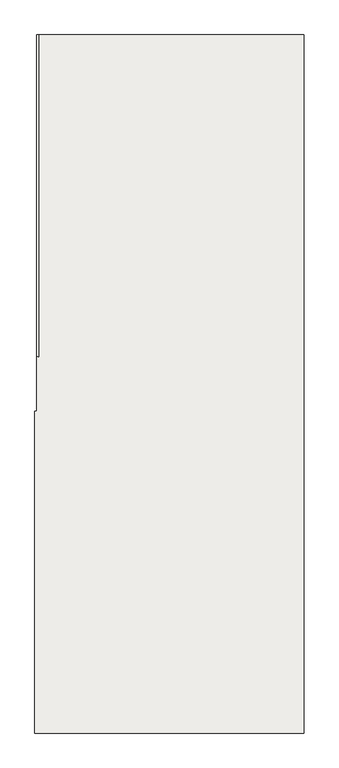
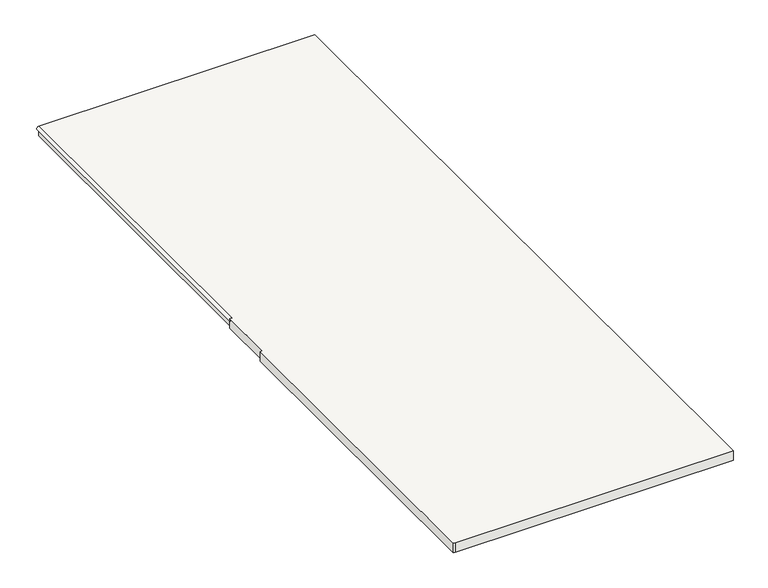
"""IFC4 building model written with IfcOpenShell, lengths in millimetres: slab geometry."""

from ifc_helpers import new_model, si_unit, frame, origin, place, context, project, spatial, circle_curve, source, transform, mapped, element, save
from ifc_brep_helpers import plane_surface, cylinder_surface, advanced_brep


def slab_de2634ce(model_context):
    return source(origin(), model_context, "Body", "AdvancedBrep", [
        advanced_brep(
        [(2237.0011137, -4486.6352742, 2086.9565217), (2237.0011137, -4486.6352742, 2066.9565217), (2237.0011137, -6137.6352742, 2066.9565217), (2227.0011137, -6137.6352742, 2076.9565217), (2237.0011137, -6137.6352742, 2086.9565217), (2227.0011137, -6137.6352742, 2086.9565217), (2227.0011137, -6414.821978, 2086.9565217), (2217.0011137, -6414.821978, 2086.9565217), (2217.0011137, -8065.821978, 2086.9565217), (2227.0011137, -8065.821978, 2086.9565217), (3598.1511137, -8065.821978, 2086.9565217), (3598.1511137, -4486.6352742, 2086.9565217), (2237.0011137, -6137.6352742, 2036.9565217), (2237.0011137, -4486.6352742, 2036.9565217), (3598.1511137, -4486.6352742, 2036.9565217), (3598.1511137, -8065.821978, 2036.9565217), (2227.0011137, -8065.821978, 2036.9565217), (2217.0011137, -8065.821978, 2036.9565217), (2217.0011137, -6414.821978, 2036.9565217), (2227.0011137, -6414.821978, 2036.9565217), (2227.0011137, -6137.6352742, 2036.9565217)],
        [
            (0, 1, circle_curve(frame((2237.0011137, -4486.6352742, 2076.9565217), z_axis=(0.0, -1.0, 0.0), x_axis=(1.0, 0.0, 0.0)), 10.0)),
            (1, 2),
            (2, 3, circle_curve(frame((2237.0011137, -6137.6352742, 2076.9565217), z_axis=(0.0, 1.0, 0.0), x_axis=(1.0, 0.0, 0.0)), 10.0)),
            (3, 4, circle_curve(frame((2237.0011137, -6137.6352742, 2076.9565217), z_axis=(0.0, 1.0, 0.0), x_axis=(1.0, 0.0, 0.0)), 10.0)),
            (4, 0),
            (4, 5),
            (5, 6),
            (6, 7),
            (7, 8),
            (8, 9),
            (9, 10),
            (10, 11),
            (11, 0),
            (12, 13),
            (13, 14),
            (14, 15),
            (15, 16),
            (16, 17),
            (17, 18),
            (18, 19),
            (19, 20),
            (20, 12),
            (12, 2),
            (1, 13),
            (3, 5),
            (20, 3),
            (19, 6),
            (18, 7),
            (17, 8),
            (16, 9),
            (15, 10),
            (14, 11),
        ],
        [
            cylinder_surface(frame((2237.0011137, -6137.6352742, 2076.9565217), z_axis=(0.0, -1.0, 0.0), x_axis=(1.0, 0.0, 0.0)), 10.0),
            plane_surface(frame((2237.0011137, -4486.6352742, 2086.9565217), z_axis=(0.0, 0.0, 1.0), x_axis=(0.0, -1.0, 0.0))),
            plane_surface(frame((2237.0011137, -4486.6352742, 2036.9565217), z_axis=(0.0, 0.0, -1.0), x_axis=(0.0, 1.0, 0.0))),
            plane_surface(frame((2237.0011137, -4486.6352742, 2086.9565217), z_axis=(-1.0, 0.0, 0.0), x_axis=(0.0, 0.0, -1.0))),
            plane_surface(frame((2237.0011137, -6137.6352742, 2086.9565217), z_axis=(0.0, 1.0, 0.0), x_axis=(0.0, 0.0, -1.0))),
            plane_surface(frame((2227.0011137, -6137.6352742, 2086.9565217), z_axis=(-1.0, 0.0, 0.0), x_axis=(0.0, 0.0, -1.0))),
            plane_surface(frame((2227.0011137, -6414.821978, 2086.9565217), z_axis=(0.0, 1.0, 0.0), x_axis=(0.0, 0.0, -1.0))),
            plane_surface(frame((2217.0011137, -6414.821978, 2086.9565217), z_axis=(-1.0, 0.0, 0.0), x_axis=(0.0, 0.0, -1.0))),
            plane_surface(frame((2217.0011137, -8065.821978, 2086.9565217), z_axis=(0.0, -1.0, 0.0), x_axis=(0.0, 0.0, -1.0))),
            plane_surface(frame((2227.0011137, -8065.821978, 2086.9565217), z_axis=(0.0, -1.0, 0.0), x_axis=(0.0, 0.0, -1.0))),
            plane_surface(frame((3598.1511137, -8065.821978, 2086.9565217), z_axis=(1.0, 0.0, 0.0), x_axis=(0.0, 0.0, -1.0))),
            plane_surface(frame((3598.1511137, -4486.6352742, 2086.9565217), z_axis=(0.0, 1.0, 0.0), x_axis=(0.0, 0.0, -1.0))),
        ],
        [
            (0, [[1, 2, 3, 4, 5]]),
            (1, [[6, 7, 8, 9, 10, 11, 12, 13, -5]]),
            (2, [[14, 15, 16, 17, 18, 19, 20, 21, 22]]),
            (3, [[-14, 23, -2, 24]]),
            (4, [[-6, -4, 25]]),
            (4, [[-22, 26, -3, -23]]),
            (5, [[-7, -25, -26, -21, 27]]),
            (6, [[-8, -27, -20, 28]]),
            (7, [[-9, -28, -19, 29]]),
            (8, [[-10, -29, -18, 30]]),
            (9, [[-11, -30, -17, 31]]),
            (10, [[-12, -31, -16, 32]]),
            (11, [[-13, -32, -15, -24, -1]]),
        ],
    ),
    ])


if __name__ == "__main__":
    model = new_model("IFC4")
    model_context = context("Model", 3, world=origin())
    ifc_project = project(units=[si_unit("LENGTHUNIT", "METRE", prefix="MILLI")], contexts=[model_context])
    site = spatial("IfcSite", under=ifc_project)
    building = spatial("IfcBuilding", under=site)
    placement = place(None, origin())
    slab_shape = slab_de2634ce(model_context)
    element("IfcSlab", 1, at=placement, inside=building, context=model_context, shape_type="MappedRepresentation", body=[
        mapped(slab_shape, transform((0.0, 0.0, 0.0), x_axis=(1.0, 0.0, 0.0), y_axis=(0.0, 1.0, 0.0), z_axis=(0.0, 0.0, 1.0))),
    ])
    save(model, "model.ifc")

# Revit data of these elements
# Element 1 (IfcSlab)
#   Materials on its faces: "Oak Flooring"
# Materials
#   "Oak Flooring": class "Wood", colour RGB 212 179 113, transparency 0, Description = "Quercus Rubra", Cost = 0
